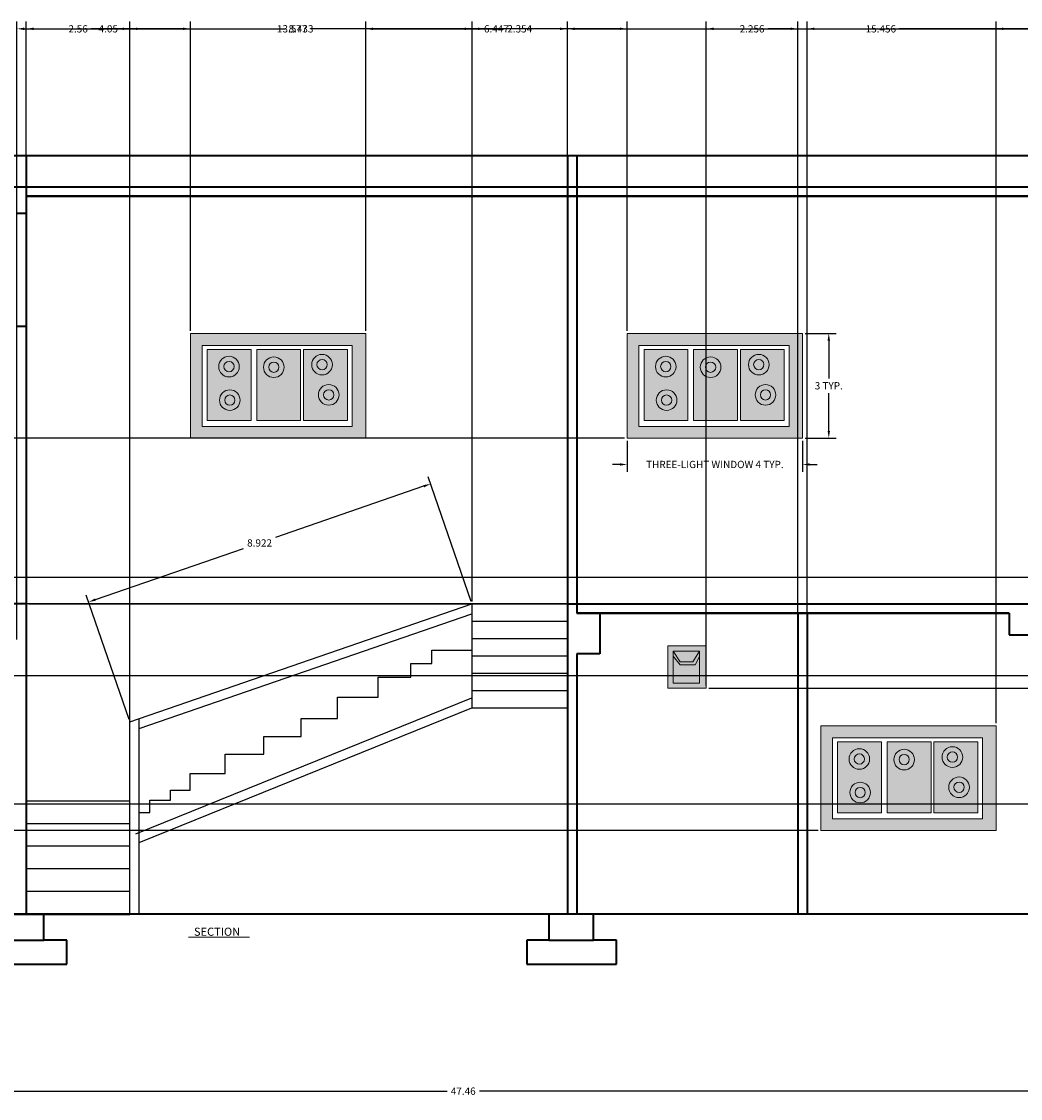
# Model space of a CAD drawing. Units: metres. Extents: x 1976.6 to 2045, y 823.7 to 850.3.
# Tile 2 of 3: x 2006.5 to 2031.2, y 823.7 to 850.3. Entities that reach past the tile are written whole.
import ezdxf

# ---------------------------------------------------------------- set-up
doc = ezdxf.new("R2010")
doc.units = ezdxf.units.M
for name, color, linetype, lineweight in [('A-ANNO-DIMS', 2, 'Continuous', 18), ('A-ANNO-TEXT', 7, 'Continuous', 18), ('A-COLS', 1, 'Continuous', 35), ('A-FLOR', 7, 'Continuous', 35), ('A-FLOR-STRS', 7, 'Continuous', 25), ('A-GLAZ', 4, 'Continuous', 18), ('A-ROOF', 7, 'Continuous', 35), ('A-WALL', 7, 'Continuous', 35), ('A-WALL-PRPT', 7, 'Continuous', 35), ('S-BEAM', 1, 'Continuous', 35), ('S-FNDN', 1, 'Continuous', 35)]:
    doc.layers.add(name, color=color, linetype=linetype, lineweight=lineweight)
doc.styles.get("Standard").update_dxf_attribs({"font": 'arial.ttf'})
doc.dimstyles.get("Standard").update_dxf_attribs({"dimtxt": 0.18, "dimasz": 0.18, "dimexe": 0.18, "dimexo": 0.0625, "dimgap": 0.09, "dimtad": 0, "dimtih": 1, "dimtoh": 1, "dimdec": 4, "dimzin": 0, "dimdsep": 46, "dimtxsty": 'Standard', "dimcen": 0.09, "dimadec": 0, "dimazin": 0, "dimtfac": 1, "dimtdec": 4, "dimtofl": 0, "dimtmove": 0, "dimatfit": 3, "dimfxl": 1, "dimtolj": 1, "dimtzin": 0, "dimarcsym": 0})

# ---------------------------------------------------------------- blocks, each defined once
blk = doc.blocks.new('WIN-THREE-LIGHT-ORNAMENTAL')
h = blk.add_hatch(color=256)
h.dxf.hatch_style = 1
h.paths.add_polyline_path([(4.324, 2.582), (0, 2.582), (0, 0), (4.324, 0)])
h.paths.add_polyline_path([(0.291, 2.284), (3.992, 2.284), (3.992, 0.289), (0.291, 0.289)], flags=16)
h.paths.add_polyline_path([(0.416, 2.189), (1.499, 2.189), (1.499, 0.436), (0.416, 0.436)], flags=0)
h.paths.add_polyline_path([(1.636, 2.189), (2.72, 2.189), (2.72, 0.436), (1.636, 0.436)], flags=0)
h.paths.add_polyline_path([(2.792, 2.189), (3.875, 2.189), (3.875, 0.436), (2.792, 0.436)], flags=0)
h = blk.add_hatch(color=256)
h.dxf.hatch_style = 1
h.paths.add_polyline_path([(1.499, 2.189), (0.416, 2.189), (0.416, 0.436), (1.499, 0.436)])
h.paths.add_polyline_path([(2.72, 2.189), (1.636, 2.189), (1.636, 0.436), (2.72, 0.436)])
h.paths.add_polyline_path([(3.875, 2.189), (2.792, 2.189), (2.792, 0.436), (3.875, 0.436)])
h = blk.add_hatch(color=256)
h.dxf.hatch_style = 1
h.paths.add_polyline_path([(1.207, 1.764, 1), (0.699, 1.764, 1)])
h.paths.add_polyline_path([(0.826, 1.764, -1), (1.08, 1.764, -1)], flags=16)
h = blk.add_hatch(color=256)
h.dxf.hatch_style = 1
h.paths.add_polyline_path([(2.312, 1.749, 1), (1.804, 1.749, 1)])
h.paths.add_polyline_path([(1.931, 1.749, -1), (2.186, 1.749, -1)], flags=16)
h = blk.add_hatch(color=256)
h.dxf.hatch_style = 1
h.paths.add_polyline_path([(3.501, 1.812, 1), (2.993, 1.812, 1)])
h.paths.add_polyline_path([(3.12, 1.812, -1), (3.374, 1.812, -1)], flags=16)
h = blk.add_hatch(color=256)
h.dxf.hatch_style = 1
h.paths.add_polyline_path([(1.227, 0.938, 1), (0.719, 0.938, 1)])
h.paths.add_polyline_path([(0.846, 0.938, -1), (1.1, 0.938, -1)], flags=16)
h = blk.add_hatch(color=256)
h.dxf.hatch_style = 1
h.paths.add_polyline_path([(2.366, 0.938, 1), (1.858, 0.938, 1)])
h.paths.add_polyline_path([(1.985, 0.938, -1), (2.239, 0.938, -1)], flags=16)
h = blk.add_hatch(color=256)
h.dxf.hatch_style = 1
h.paths.add_polyline_path([(3.666, 1.067, 1), (3.158, 1.067, 1)])
h.paths.add_polyline_path([(3.285, 1.067, -1), (3.539, 1.067, -1)], flags=16)
for points in [[(0, 2.582), (4.324, 2.582), (4.324, 0), (0, 0)], [(0.291, 2.284), (3.992, 2.284), (3.992, 0.289), (0.291, 0.289)], [(0.416, 2.189), (1.499, 2.189), (1.499, 0.436), (0.416, 0.436)], [(1.636, 2.189), (2.72, 2.189), (2.72, 0.436), (1.636, 0.436)], [(2.792, 2.189), (3.875, 2.189), (3.875, 0.436), (2.792, 0.436)]]:
    blk.add_lwpolyline(points, close=True)
for centre, radius in [((0.953, 1.764), 0.254), ((0.953, 1.764), 0.127), ((2.058, 1.749), 0.254), ((2.058, 1.749), 0.127), ((3.247, 1.812), 0.254), ((3.247, 1.812), 0.127), ((0.973, 0.938), 0.254), ((0.973, 0.938), 0.127), ((3.412, 1.067), 0.254), ((3.412, 1.067), 0.127)]:
    blk.add_circle(centre, radius)
blk = doc.blocks.new('WIN-VENT')
h = blk.add_hatch(color=256)
h.dxf.hatch_style = 1
h.paths.add_polyline_path([(0.783, 0.781), (0.783, 0.912), (0.616, 0.651), (0.305, 0.651), (0.133, 0.912), (0.133, 0.788), (0.305, 0.57), (0.677, 0.57)], flags=0)
h.paths.add_polyline_path([(0.95, 1.042), (0, 1.042), (0, 0), (0.95, 0)])
h.paths.add_polyline_path([(0.783, 0.912), (0.783, 0.125), (0.133, 0.125), (0.133, 0.912)], flags=16)
h.paths.add_polyline_path([(0.783, 0.781), (0.783, 0.912), (0.133, 0.912), (0.133, 0.788), (0.305, 0.57), (0.677, 0.57)], flags=0)
h = blk.add_hatch(color=256)
h.dxf.hatch_style = 1
h.paths.add_polyline_path([(0.783, 0.781), (0.783, 0.912), (0.616, 0.651), (0.305, 0.651), (0.133, 0.912), (0.133, 0.788), (0.305, 0.57), (0.677, 0.57)])
h = blk.add_hatch(color=256)
h.dxf.hatch_style = 1
h.paths.add_polyline_path([(0.133, 0.912), (0.305, 0.651), (0.616, 0.651), (0.783, 0.912)])
h.paths.add_polyline_path([(0.783, 0.125), (0.783, 0.781), (0.677, 0.57), (0.305, 0.57), (0.133, 0.788), (0.133, 0.125)])
for p, q in [((0.133, 0.912), (0.305, 0.651)), ((0.133, 0.912), (0.133, 0.788)), ((0.616, 0.651), (0.783, 0.912)), ((0.133, 0.788), (0.305, 0.57)), ((0.305, 0.651), (0.616, 0.651)), ((0.305, 0.57), (0.677, 0.57)), ((0.677, 0.57), (0.783, 0.781))]:
    blk.add_line(p, q)
for points in [[(0, 1.042), (0.95, 1.042), (0.95, 0), (0, 0)], [(0.133, 0.912), (0.783, 0.912), (0.783, 0.125), (0.133, 0.125)]]:
    blk.add_lwpolyline(points, close=True)
blk = doc.blocks.new('FNDN-STEPPED-PAD')
for p, q in [((0.547, 1.235), (0.547, 0.59)), ((1.641, 0.59), (1.641, 1.235)), ((0.547, 0.59), (0, 0.59)), ((0, 0.59), (0, 0)), ((0.547, 0.59), (1.641, 0.59)), ((2.209, 0.59), (1.641, 0.59)), ((2.209, 0), (2.209, 0.59)), ((0, 0), (2.209, 0))]:
    blk.add_line(p, q)
blk = doc.blocks.new('*D8')
at = {"layer": 'A-ANNO-DIMS', "color": 0, "lineweight": -2, "transparency": 16777216}
for p, q in [((2021.467, 839.959), (2021.467, 839.193)), ((2025.79, 839.959), (2025.79, 839.193)), ((2021.287, 839.373), (2021.107, 839.373)), ((2025.97, 839.373), (2026.15, 839.373))]:
    blk.add_line(p, q, dxfattribs=at)
at = {"layer": 'A-ANNO-DIMS', "color": 0, "transparency": 16777216}
for points in [[(2021.287, 839.403), (2021.287, 839.343), (2021.467, 839.373)], [(2025.97, 839.403), (2025.97, 839.343), (2025.79, 839.373)]]:
    blk.add_solid(points, dxfattribs=at)
at = {"layer": 'Defpoints', "color": 0, "transparency": 16777216}
for p in [(2021.467, 840.022), (2025.79, 840.022), (2025.79, 839.373)]:
    blk.add_point(p, dxfattribs=at)
at = {"layer": 'A-ANNO-DIMS', "color": 0, "transparency": 16777216, "insert": (2023.629, 839.373), "char_height": 0.18, "attachment_point": 5}
blk.add_mtext('\\A1;THREE-LIGHT WINDOW 4 TYP.', dxfattribs=at)
blk = doc.blocks.new('*D9')
at = {"layer": 'A-ANNO-DIMS', "color": 0, "lineweight": -2, "transparency": 16777216}
for p, q in [((2025.853, 842.604), (2026.619, 842.604)), ((2026.439, 842.424), (2026.439, 841.495)), ((2026.439, 840.202), (2026.439, 841.131)), ((2025.853, 840.022), (2026.619, 840.022))]:
    blk.add_line(p, q, dxfattribs=at)
at = {"layer": 'A-ANNO-DIMS', "color": 0, "transparency": 16777216}
for points in [[(2026.409, 842.424), (2026.469, 842.424), (2026.439, 842.604)], [(2026.409, 840.202), (2026.469, 840.202), (2026.439, 840.022)]]:
    blk.add_solid(points, dxfattribs=at)
at = {"layer": 'Defpoints', "color": 0, "transparency": 16777216}
for p in [(2025.79, 842.604), (2026.439, 842.604), (2025.79, 840.022)]:
    blk.add_point(p, dxfattribs=at)
at = {"layer": 'A-ANNO-DIMS', "color": 0, "transparency": 16777216, "insert": (2026.439, 841.313), "char_height": 0.18, "attachment_point": 5}
blk.add_mtext('\\A1;3 TYP.', dxfattribs=at)
blk = doc.blocks.new('*D16')
at = {"layer": 'A-ANNO-DIMS', "color": 0, "lineweight": -2, "transparency": 16777216}
for p, q in [((1993.695, 826.987), (1993.695, 823.74)), ((2041.154, 826.987), (2041.154, 823.74)), ((1993.875, 823.92), (2017.027, 823.92)), ((2040.974, 823.92), (2017.822, 823.92))]:
    blk.add_line(p, q, dxfattribs=at)
at = {"layer": 'A-ANNO-DIMS', "color": 0, "transparency": 16777216}
for points in [[(1993.875, 823.95), (1993.875, 823.89), (1993.695, 823.92)], [(2040.974, 823.95), (2040.974, 823.89), (2041.154, 823.92)]]:
    blk.add_solid(points, dxfattribs=at)
at = {"layer": 'Defpoints', "color": 0, "transparency": 16777216}
for p in [(1993.695, 827.05), (2041.154, 827.05), (2041.154, 823.92)]:
    blk.add_point(p, dxfattribs=at)
at = {"layer": 'A-ANNO-DIMS', "color": 0, "transparency": 16777216, "insert": (2017.425, 823.92), "char_height": 0.18, "attachment_point": 5}
blk.add_mtext('\\A1;47.46', dxfattribs=at)
blk = doc.blocks.new('*D20')
at = {"layer": 'A-ANNO-DIMS', "color": 0, "lineweight": -2, "transparency": 16777216}
for p, q in [((2006.418, 847.047), (2006.418, 850.295)), ((2019.995, 847.047), (2019.995, 850.295)), ((2006.598, 850.115), (2012.751, 850.115)), ((2019.815, 850.115), (2013.661, 850.115))]:
    blk.add_line(p, q, dxfattribs=at)
at = {"layer": 'A-ANNO-DIMS', "color": 0, "transparency": 16777216}
for points in [[(2006.598, 850.145), (2006.598, 850.085), (2006.418, 850.115)], [(2019.815, 850.145), (2019.815, 850.085), (2019.995, 850.115)]]:
    blk.add_solid(points, dxfattribs=at)
at = {"layer": 'Defpoints', "color": 0, "transparency": 16777216}
for p in [(2019.995, 850.115), (2006.418, 846.985), (2019.995, 846.985)]:
    blk.add_point(p, dxfattribs=at)
at = {"layer": 'A-ANNO-DIMS', "color": 0, "transparency": 16777216, "insert": (2013.206, 850.115), "char_height": 0.18, "attachment_point": 5}
blk.add_mtext('\\A1;13.577', dxfattribs=at)
blk = doc.blocks.new('*D21')
at = {"layer": 'A-ANNO-DIMS', "color": 0, "lineweight": -2, "transparency": 16777216}
for p, q in [((2019.995, 847.047), (2019.995, 850.295)), ((2035.451, 847.047), (2035.451, 850.295)), ((2020.175, 850.115), (2027.268, 850.115)), ((2035.271, 850.115), (2028.178, 850.115))]:
    blk.add_line(p, q, dxfattribs=at)
at = {"layer": 'A-ANNO-DIMS', "color": 0, "transparency": 16777216}
for points in [[(2020.175, 850.145), (2020.175, 850.085), (2019.995, 850.115)], [(2035.271, 850.145), (2035.271, 850.085), (2035.451, 850.115)]]:
    blk.add_solid(points, dxfattribs=at)
at = {"layer": 'Defpoints', "color": 0, "transparency": 16777216}
for p in [(2035.451, 850.115), (2019.995, 846.985), (2035.451, 846.985)]:
    blk.add_point(p, dxfattribs=at)
at = {"layer": 'A-ANNO-DIMS', "color": 0, "transparency": 16777216, "insert": (2027.723, 850.115), "char_height": 0.18, "attachment_point": 5}
blk.add_mtext('\\A1;15.456', dxfattribs=at)
blk = doc.blocks.new('*D23')
at = {"layer": 'A-ANNO-DIMS', "color": 0, "lineweight": -2, "transparency": 16777216}
for p, q in [((2006.71, 835.935), (2044.464, 835.935)), ((2044.284, 835.755), (2044.284, 832.292)), ((2044.284, 828.465), (2044.284, 831.928)), ((2006.71, 828.285), (2044.464, 828.285))]:
    blk.add_line(p, q, dxfattribs=at)
at = {"layer": 'A-ANNO-DIMS', "color": 0, "transparency": 16777216}
for points in [[(2044.254, 835.755), (2044.314, 835.755), (2044.284, 835.935)], [(2044.254, 828.465), (2044.314, 828.465), (2044.284, 828.285)]]:
    blk.add_solid(points, dxfattribs=at)
at = {"layer": 'Defpoints', "color": 0, "transparency": 16777216}
for p in [(2006.648, 835.935), (2044.284, 835.935), (2006.648, 828.285)]:
    blk.add_point(p, dxfattribs=at)
at = {"layer": 'A-ANNO-DIMS', "color": 0, "transparency": 16777216, "insert": (2044.284, 832.11), "char_height": 0.18, "attachment_point": 5}
blk.add_mtext('\\A1;7.65', dxfattribs=at)
blk = doc.blocks.new('*D26')
at = {"layer": 'A-ANNO-DIMS', "color": 0, "lineweight": -2, "transparency": 16777216}
for p, q in [((2006.648, 828.347), (2006.648, 850.295)), ((2009.207, 828.347), (2009.207, 850.295)), ((2006.828, 850.115), (2007.602, 850.115)), ((2009.027, 850.115), (2008.253, 850.115))]:
    blk.add_line(p, q, dxfattribs=at)
at = {"layer": 'A-ANNO-DIMS', "color": 0, "transparency": 16777216}
for points in [[(2006.828, 850.145), (2006.828, 850.085), (2006.648, 850.115)], [(2009.027, 850.145), (2009.027, 850.085), (2009.207, 850.115)]]:
    blk.add_solid(points, dxfattribs=at)
at = {"layer": 'Defpoints', "color": 0, "transparency": 16777216}
for p in [(2009.207, 850.115), (2006.648, 828.285), (2009.207, 828.285)]:
    blk.add_point(p, dxfattribs=at)
at = {"layer": 'A-ANNO-DIMS', "color": 0, "transparency": 16777216, "insert": (2007.928, 850.115), "char_height": 0.18, "attachment_point": 5}
blk.add_mtext('\\A1;2.56', dxfattribs=at)
blk = doc.blocks.new('*D27')
at = {"layer": 'A-ANNO-DIMS', "color": 0, "lineweight": -2, "transparency": 16777216}
for p, q in [((2009.207, 833.086), (2009.207, 850.295)), ((2017.641, 835.997), (2017.641, 850.295)), ((2009.387, 850.115), (2013.03, 850.115)), ((2017.461, 850.115), (2013.818, 850.115))]:
    blk.add_line(p, q, dxfattribs=at)
at = {"layer": 'A-ANNO-DIMS', "color": 0, "transparency": 16777216}
for points in [[(2009.387, 850.145), (2009.387, 850.085), (2009.207, 850.115)], [(2017.461, 850.145), (2017.461, 850.085), (2017.641, 850.115)]]:
    blk.add_solid(points, dxfattribs=at)
at = {"layer": 'Defpoints', "color": 0, "transparency": 16777216}
for p in [(2017.641, 850.115), (2017.641, 835.935), (2009.207, 833.023)]:
    blk.add_point(p, dxfattribs=at)
at = {"layer": 'A-ANNO-DIMS', "color": 0, "transparency": 16777216, "insert": (2013.424, 850.115), "char_height": 0.18, "attachment_point": 5}
blk.add_mtext('\\A1;8.433', dxfattribs=at)
blk = doc.blocks.new('*D28')
at = {"layer": 'A-ANNO-DIMS', "color": 0, "lineweight": -2, "transparency": 16777216}
for p, q in [((2017.62, 835.994), (2016.561, 839.064)), ((2016.449, 838.835), (2012.796, 837.573)), ((2008.356, 836.041), (2012.01, 837.302)), ((2009.187, 833.082), (2008.127, 836.152))]:
    blk.add_line(p, q, dxfattribs=at)
at = {"layer": 'A-ANNO-DIMS', "color": 0, "transparency": 16777216}
for points in [[(2016.439, 838.863), (2016.459, 838.806), (2016.619, 838.893)], [(2008.346, 836.069), (2008.366, 836.012), (2008.186, 835.982)]]:
    blk.add_solid(points, dxfattribs=at)
at = {"layer": 'Defpoints', "color": 0, "transparency": 16777216}
for p in [(2016.619, 838.893), (2017.641, 835.935), (2009.207, 833.023)]:
    blk.add_point(p, dxfattribs=at)
at = {"layer": 'A-ANNO-DIMS', "color": 0, "transparency": 16777216, "insert": (2012.403, 837.438), "char_height": 0.18, "attachment_point": 5}
blk.add_mtext('\\A1;8.922', dxfattribs=at)
blk = doc.blocks.new('*D29')
at = {"layer": 'A-ANNO-DIMS', "color": 0, "lineweight": -2, "transparency": 16777216}
for p, q in [((2017.641, 835.997), (2017.641, 850.295)), ((2019.995, 835.997), (2019.995, 850.295)), ((2017.821, 850.115), (2018.423, 850.115)), ((2019.815, 850.115), (2019.213, 850.115))]:
    blk.add_line(p, q, dxfattribs=at)
at = {"layer": 'A-ANNO-DIMS', "color": 0, "transparency": 16777216}
for points in [[(2017.821, 850.145), (2017.821, 850.085), (2017.641, 850.115)], [(2019.815, 850.145), (2019.815, 850.085), (2019.995, 850.115)]]:
    blk.add_solid(points, dxfattribs=at)
at = {"layer": 'Defpoints', "color": 0, "transparency": 16777216}
for p in [(2019.995, 850.115), (2017.641, 835.935), (2019.995, 835.935)]:
    blk.add_point(p, dxfattribs=at)
at = {"layer": 'A-ANNO-DIMS', "color": 0, "transparency": 16777216, "insert": (2018.818, 850.115), "char_height": 0.18, "attachment_point": 5}
blk.add_mtext('\\A1;2.354', dxfattribs=at)
blk = doc.blocks.new('*D30')
at = {"layer": 'A-ANNO-DIMS', "color": 0, "lineweight": -2, "transparency": 16777216}
for p, q in [((2025.906, 828.347), (2025.906, 850.295)), ((2039.878, 828.347), (2039.878, 850.295)), ((2026.086, 850.115), (2032.437, 850.115)), ((2039.698, 850.115), (2033.346, 850.115))]:
    blk.add_line(p, q, dxfattribs=at)
at = {"layer": 'A-ANNO-DIMS', "color": 0, "transparency": 16777216}
for points in [[(2026.086, 850.145), (2026.086, 850.085), (2025.906, 850.115)], [(2039.698, 850.145), (2039.698, 850.085), (2039.878, 850.115)]]:
    blk.add_solid(points, dxfattribs=at)
at = {"layer": 'Defpoints', "color": 0, "transparency": 16777216}
for p in [(2039.878, 850.115), (2025.906, 828.285), (2039.878, 828.285)]:
    blk.add_point(p, dxfattribs=at)
at = {"layer": 'A-ANNO-DIMS', "color": 0, "transparency": 16777216, "insert": (2032.892, 850.115), "char_height": 0.18, "attachment_point": 5}
blk.add_mtext('\\A1;13.972', dxfattribs=at)
blk = doc.blocks.new('*D32')
at = {"layer": 'A-ANNO-DIMS', "color": 0, "lineweight": -2, "transparency": 16777216}
for p, q in [((1997.363, 831.006), (2044.464, 831.006)), ((2044.284, 830.826), (2044.284, 829.826)), ((2044.284, 828.465), (2044.284, 829.465)), ((1994.937, 828.285), (2044.464, 828.285))]:
    blk.add_line(p, q, dxfattribs=at)
at = {"layer": 'A-ANNO-DIMS', "color": 0, "transparency": 16777216}
for points in [[(2044.254, 830.826), (2044.314, 830.826), (2044.284, 831.006)], [(2044.254, 828.465), (2044.314, 828.465), (2044.284, 828.285)]]:
    blk.add_solid(points, dxfattribs=at)
at = {"layer": 'Defpoints', "color": 0, "transparency": 16777216}
for p in [(1997.3, 831.006), (1994.875, 828.285), (2044.284, 828.285)]:
    blk.add_point(p, dxfattribs=at)
at = {"layer": 'A-ANNO-DIMS', "color": 0, "transparency": 16777216, "insert": (2044.284, 829.645), "char_height": 0.18, "attachment_point": 5}
blk.add_mtext('\\A1;2.721', dxfattribs=at)
blk = doc.blocks.new('*D36')
at = {"layer": 'A-ANNO-DIMS', "color": 0, "lineweight": -2, "transparency": 16777216}
for p, q in [((2005.307, 834.228), (2005.307, 850.295)), ((2006.418, 835.06), (2006.418, 850.295)), ((2005.127, 850.115), (2004.947, 850.115)), ((2006.598, 850.115), (2006.778, 850.115))]:
    blk.add_line(p, q, dxfattribs=at)
at = {"layer": 'A-ANNO-DIMS', "color": 0, "transparency": 16777216}
for points in [[(2005.127, 850.145), (2005.127, 850.085), (2005.307, 850.115)], [(2006.598, 850.145), (2006.598, 850.085), (2006.418, 850.115)]]:
    blk.add_solid(points, dxfattribs=at)
at = {"layer": 'Defpoints', "color": 0, "transparency": 16777216}
for p in [(2006.418, 850.115), (2006.418, 834.998), (2005.307, 834.166)]:
    blk.add_point(p, dxfattribs=at)
at = {"layer": 'A-ANNO-DIMS', "color": 0, "transparency": 16777216, "insert": (2005.862, 850.115), "char_height": 0.18, "attachment_point": 5}
blk.add_mtext('\\A1;1.11', dxfattribs=at)
blk = doc.blocks.new('*D38')
at = {"layer": 'A-ANNO-DIMS', "color": 0, "lineweight": -2, "transparency": 16777216}
for p, q in [((2005.369, 834.166), (2044.464, 834.166)), ((2044.284, 833.986), (2044.284, 831.407)), ((2044.284, 828.465), (2044.284, 831.043)), ((2005.369, 828.285), (2044.464, 828.285))]:
    blk.add_line(p, q, dxfattribs=at)
at = {"layer": 'A-ANNO-DIMS', "color": 0, "transparency": 16777216}
for points in [[(2044.254, 833.986), (2044.314, 833.986), (2044.284, 834.166)], [(2044.254, 828.465), (2044.314, 828.465), (2044.284, 828.285)]]:
    blk.add_solid(points, dxfattribs=at)
at = {"layer": 'Defpoints', "color": 0, "transparency": 16777216}
for p in [(2005.307, 834.166), (2005.307, 828.285), (2044.284, 828.285)]:
    blk.add_point(p, dxfattribs=at)
at = {"layer": 'A-ANNO-DIMS', "color": 0, "transparency": 16777216, "insert": (2044.284, 831.225), "char_height": 0.18, "attachment_point": 5}
blk.add_mtext('\\A1;5.881', dxfattribs=at)
blk = doc.blocks.new('*D39')
at = {"layer": 'A-ANNO-DIMS', "color": 0, "lineweight": -2, "transparency": 16777216}
for p, q in [((2006.648, 842.847), (2006.648, 850.295)), ((2010.696, 842.666), (2010.696, 850.295)), ((2006.828, 850.115), (2008.344, 850.115)), ((2010.516, 850.115), (2009, 850.115))]:
    blk.add_line(p, q, dxfattribs=at)
at = {"layer": 'A-ANNO-DIMS', "color": 0, "transparency": 16777216}
for points in [[(2006.828, 850.145), (2006.828, 850.085), (2006.648, 850.115)], [(2010.516, 850.145), (2010.516, 850.085), (2010.696, 850.115)]]:
    blk.add_solid(points, dxfattribs=at)
at = {"layer": 'Defpoints', "color": 0, "transparency": 16777216}
for p in [(2010.696, 850.115), (2006.648, 842.785), (2010.696, 842.604)]:
    blk.add_point(p, dxfattribs=at)
at = {"layer": 'A-ANNO-DIMS', "color": 0, "transparency": 16777216, "insert": (2008.672, 850.115), "char_height": 0.18, "attachment_point": 5}
blk.add_mtext('\\A1;4.05', dxfattribs=at)
blk = doc.blocks.new('*D40')
at = {"layer": 'A-ANNO-DIMS', "color": 0, "lineweight": -2, "transparency": 16777216}
for p, q in [((2015.02, 842.666), (2015.02, 850.295)), ((2021.467, 842.666), (2021.467, 850.295)), ((2015.2, 850.115), (2017.849, 850.115)), ((2021.287, 850.115), (2018.638, 850.115))]:
    blk.add_line(p, q, dxfattribs=at)
at = {"layer": 'A-ANNO-DIMS', "color": 0, "transparency": 16777216}
for points in [[(2015.2, 850.145), (2015.2, 850.085), (2015.02, 850.115)], [(2021.287, 850.145), (2021.287, 850.085), (2021.467, 850.115)]]:
    blk.add_solid(points, dxfattribs=at)
at = {"layer": 'Defpoints', "color": 0, "transparency": 16777216}
for p in [(2021.467, 850.115), (2015.02, 842.604), (2021.467, 842.604)]:
    blk.add_point(p, dxfattribs=at)
at = {"layer": 'A-ANNO-DIMS', "color": 0, "transparency": 16777216, "insert": (2018.243, 850.115), "char_height": 0.18, "attachment_point": 5}
blk.add_mtext('\\A1;6.447', dxfattribs=at)
blk = doc.blocks.new('*D41')
at = {"layer": 'A-ANNO-DIMS', "color": 0, "lineweight": -2, "transparency": 16777216}
for p, q in [((2026.178, 830.345), (1986.237, 830.345)), ((1986.417, 830.165), (1986.417, 829.497)), ((1986.417, 828.465), (1986.417, 829.133)), ((2025.843, 828.285), (1986.237, 828.285))]:
    blk.add_line(p, q, dxfattribs=at)
at = {"layer": 'A-ANNO-DIMS', "color": 0, "transparency": 16777216}
for points in [[(1986.387, 830.165), (1986.447, 830.165), (1986.417, 830.345)], [(1986.387, 828.465), (1986.447, 828.465), (1986.417, 828.285)]]:
    blk.add_solid(points, dxfattribs=at)
at = {"layer": 'Defpoints', "color": 0, "transparency": 16777216}
for p in [(2026.24, 830.345), (1986.417, 828.285), (2025.906, 828.285)]:
    blk.add_point(p, dxfattribs=at)
at = {"layer": 'A-ANNO-DIMS', "color": 0, "transparency": 16777216, "insert": (1986.417, 829.315), "char_height": 0.18, "attachment_point": 5}
blk.add_mtext('\\A1;2.06', dxfattribs=at)
blk = doc.blocks.new('*D42')
at = {"layer": 'A-ANNO-DIMS', "color": 0, "lineweight": -2, "transparency": 16777216}
for p, q in [((2021.404, 840.022), (1986.237, 840.022)), ((1986.417, 839.842), (1986.417, 838.16)), ((1986.417, 836.115), (1986.417, 837.796)), ((2020.162, 835.935), (1986.237, 835.935))]:
    blk.add_line(p, q, dxfattribs=at)
at = {"layer": 'A-ANNO-DIMS', "color": 0, "transparency": 16777216}
for points in [[(1986.387, 839.842), (1986.447, 839.842), (1986.417, 840.022)], [(1986.387, 836.115), (1986.447, 836.115), (1986.417, 835.935)]]:
    blk.add_solid(points, dxfattribs=at)
at = {"layer": 'Defpoints', "color": 0, "transparency": 16777216}
for p in [(2021.467, 840.022), (1986.417, 835.935), (2020.225, 835.935)]:
    blk.add_point(p, dxfattribs=at)
at = {"layer": 'A-ANNO-DIMS', "color": 0, "transparency": 16777216, "insert": (1986.417, 837.978), "char_height": 0.18, "attachment_point": 5}
blk.add_mtext('\\A1;4.087', dxfattribs=at)
blk = doc.blocks.new('*D43')
at = {"layer": 'A-ANNO-DIMS', "color": 0, "lineweight": -2, "transparency": 16777216}
for p, q in [((2030.564, 832.99), (2030.564, 850.295)), ((2039.878, 832.797), (2039.878, 850.295)), ((2030.744, 850.115), (2034.827, 850.115)), ((2039.698, 850.115), (2035.614, 850.115))]:
    blk.add_line(p, q, dxfattribs=at)
at = {"layer": 'A-ANNO-DIMS', "color": 0, "transparency": 16777216}
for points in [[(2030.744, 850.145), (2030.744, 850.085), (2030.564, 850.115)], [(2039.698, 850.145), (2039.698, 850.085), (2039.878, 850.115)]]:
    blk.add_solid(points, dxfattribs=at)
at = {"layer": 'Defpoints', "color": 0, "transparency": 16777216}
for p in [(2039.878, 850.115), (2030.564, 832.927), (2039.878, 832.735)]:
    blk.add_point(p, dxfattribs=at)
at = {"layer": 'A-ANNO-DIMS', "color": 0, "transparency": 16777216, "insert": (2035.221, 850.115), "char_height": 0.18, "attachment_point": 5}
blk.add_mtext('\\A1;9.314', dxfattribs=at)
blk = doc.blocks.new('*D46')
at = {"layer": 'A-ANNO-DIMS', "color": 0, "lineweight": -2, "transparency": 16777216}
for p, q in [((2023.419, 833.921), (2023.419, 850.295)), ((2025.676, 828.347), (2025.676, 850.295)), ((2023.599, 850.115), (2024.152, 850.115)), ((2025.496, 850.115), (2024.943, 850.115))]:
    blk.add_line(p, q, dxfattribs=at)
at = {"layer": 'A-ANNO-DIMS', "color": 0, "transparency": 16777216}
for points in [[(2023.599, 850.145), (2023.599, 850.085), (2023.419, 850.115)], [(2025.496, 850.145), (2025.496, 850.085), (2025.676, 850.115)]]:
    blk.add_solid(points, dxfattribs=at)
at = {"layer": 'Defpoints', "color": 0, "transparency": 16777216}
for p in [(2025.676, 850.115), (2023.419, 833.859), (2025.676, 828.285)]:
    blk.add_point(p, dxfattribs=at)
at = {"layer": 'A-ANNO-DIMS', "color": 0, "transparency": 16777216, "insert": (2024.547, 850.115), "char_height": 0.18, "attachment_point": 5}
blk.add_mtext('\\A1;2.256', dxfattribs=at)
blk = doc.blocks.new('*D47')
at = {"layer": 'A-ANNO-DIMS', "color": 0, "lineweight": -2, "transparency": 16777216}
for p, q in [((2023.482, 833.859), (2044.464, 833.859)), ((2044.284, 833.679), (2044.284, 831.253)), ((2044.284, 828.465), (2044.284, 830.89)), ((2025.738, 828.285), (2044.464, 828.285))]:
    blk.add_line(p, q, dxfattribs=at)
at = {"layer": 'A-ANNO-DIMS', "color": 0, "transparency": 16777216}
for points in [[(2044.254, 833.679), (2044.314, 833.679), (2044.284, 833.859)], [(2044.254, 828.465), (2044.314, 828.465), (2044.284, 828.285)]]:
    blk.add_solid(points, dxfattribs=at)
at = {"layer": 'Defpoints', "color": 0, "transparency": 16777216}
for p in [(2023.419, 833.859), (2025.676, 828.285), (2044.284, 828.285)]:
    blk.add_point(p, dxfattribs=at)
at = {"layer": 'A-ANNO-DIMS', "color": 0, "transparency": 16777216, "insert": (2044.284, 831.072), "char_height": 0.18, "attachment_point": 5}
blk.add_mtext('\\A1;5.574', dxfattribs=at)
blk = doc.blocks.new('*D48')
at = {"layer": 'A-ANNO-DIMS', "color": 0, "lineweight": -2, "transparency": 16777216}
for p, q in [((2038.162, 836.589), (1986.237, 836.589)), ((1986.417, 836.409), (1986.417, 836.115)), ((2039.726, 835.935), (1986.237, 835.935)), ((1986.417, 835.755), (1986.237, 835.755)), ((1986.417, 835.935), (1986.417, 835.755))]:
    blk.add_line(p, q, dxfattribs=at)
at = {"layer": 'A-ANNO-DIMS', "color": 0, "transparency": 16777216}
for points in [[(1986.387, 836.409), (1986.447, 836.409), (1986.417, 836.589)], [(1986.387, 836.115), (1986.447, 836.115), (1986.417, 835.935)]]:
    blk.add_solid(points, dxfattribs=at)
at = {"layer": 'Defpoints', "color": 0, "transparency": 16777216}
for p in [(2038.224, 836.589), (1986.417, 835.935), (2039.788, 835.935)]:
    blk.add_point(p, dxfattribs=at)
at = {"layer": 'A-ANNO-DIMS', "color": 0, "transparency": 16777216, "insert": (1985.913, 835.755), "char_height": 0.18, "attachment_point": 5}
blk.add_mtext('\\A1;0.65', dxfattribs=at)

msp = doc.modelspace()

# ---------------------------------------------------------------- linework, layer by layer
at = {"layer": 'A-ANNO-TEXT'}
msp.add_line((2010.654, 827.7207), (2012.1564, 827.7207), dxfattribs=at)
at = {"layer": 'A-COLS'}
for p, q in [((2006.6479, 846.9848), (2006.6479, 835.9348)), ((2019.9947, 846.9848), (2019.9947, 835.9348)), ((2020.2247, 846.9848), (2020.2247, 835.9348)), ((2006.4179, 842.7848), (2006.6479, 842.7848)), ((2006.6479, 835.9348), (2006.6479, 828.2848)), ((2019.9947, 835.9348), (2019.9947, 828.2848)), ((2020.2247, 835.9348), (2020.2247, 835.7048)), ((2020.2247, 834.7023), (2020.2247, 828.2848))]:
    msp.add_line(p, q, dxfattribs=at)
at = {"layer": 'A-FLOR'}
for p, q in [((2006.6479, 835.9348), (1993.6952, 835.9348)), ((2019.9947, 835.9348), (2040.0184, 835.9348)), ((2020.2247, 835.7048), (2030.8908, 835.7048)), ((2020.2247, 835.7048), (2025.6756, 835.7048)), ((2020.2247, 835.7048), (2030.8908, 835.7048)), ((2030.8908, 835.7048), (2020.2247, 835.7048)), ((2040.5852, 828.2848), (1993.0497, 828.2848)), ((2040.5852, 828.2848), (1994.6446, 828.2848)), ((1994.6446, 828.2848), (2009.2074, 828.2848))]:
    msp.add_line(p, q, dxfattribs=at)
at = {"layer": 'A-FLOR-STRS'}
for p, q in [((2009.2074, 833.0232), (2017.6409, 835.9348)), ((2009.4374, 832.8593), (2017.6409, 835.6915)), ((2019.9947, 835.9348), (2017.6409, 835.9348)), ((2017.6409, 835.9348), (2017.6409, 834.0079)), ((2017.6409, 835.9348), (2019.9947, 835.9348)), ((2017.6409, 835.5072), (2019.9947, 835.5072)), ((2017.6409, 835.0795), (2019.9947, 835.0795)), ((2016.6543, 834.4682), (2016.6543, 834.794)), ((2016.6543, 834.794), (2017.6409, 834.794)), ((2017.6409, 834.6519), (2019.9947, 834.6519)), ((2016.1349, 834.1242), (2016.1349, 834.4682)), ((2016.1349, 834.4682), (2016.6543, 834.4682)), ((2015.3254, 833.6315), (2015.3254, 834.1242)), ((2015.3254, 834.1242), (2016.1349, 834.1242)), ((2017.6409, 834.2242), (2019.9947, 834.2242)), ((2017.6409, 834.0079), (2017.6409, 833.3689)), ((2009.3511, 830.2635), (2017.6409, 833.617)), ((2014.3265, 833.1102), (2014.3265, 833.6315)), ((2014.3265, 833.6315), (2015.3254, 833.6315)), ((2017.6409, 833.7966), (2019.9947, 833.7966)), ((2009.4374, 830.0503), (2017.6409, 833.3689)), ((2017.6409, 833.3689), (2019.9947, 833.3689)), ((2017.6409, 833.3689), (2019.9947, 833.3689)), ((2009.4374, 831.0722), (2009.4374, 833.1026)), ((2013.4319, 832.6633), (2013.4319, 833.1102)), ((2013.4319, 833.1102), (2014.3265, 833.1102)), ((2009.2074, 831.0722), (2009.2074, 833.0232)), ((2012.5075, 832.2313), (2012.5075, 832.6633)), ((2012.5075, 832.6633), (2013.4319, 832.6633)), ((2011.5533, 831.7546), (2011.5533, 832.2313)), ((2011.5533, 832.2313), (2012.5075, 832.2313)), ((2010.6924, 831.3434), (2010.6924, 831.7546)), ((2010.6924, 831.7546), (2011.5533, 831.7546)), ((2010.2088, 831.0931), (2010.2088, 831.3434)), ((2010.2088, 831.3434), (2010.6924, 831.3434)), ((2009.2074, 831.0722), (2006.6479, 831.0722)), ((2009.2074, 831.0722), (2008.9769, 831.0722)), ((2009.2074, 830.984), (2009.2074, 831.0722)), ((2009.2074, 828.2848), (2009.2074, 830.984)), ((2009.4374, 828.2848), (2009.4374, 831.0722)), ((2009.4374, 830.2984), (2009.4374, 831.0722)), ((2009.6963, 830.7879), (2009.6963, 831.0931)), ((2009.6963, 831.0931), (2010.2088, 831.0931)), ((2009.4374, 830.2984), (2009.4374, 830.7879)), ((2009.4374, 830.7879), (2009.6963, 830.7879)), ((2009.2074, 830.5147), (2006.6479, 830.5147)), ((2009.2074, 829.9572), (2006.6479, 829.9572)), ((2009.2074, 829.3998), (2009.2074, 829.9572)), ((2009.2074, 829.3998), (2006.6479, 829.3998)), ((2009.2074, 828.8423), (2006.6479, 828.8423)), ((2009.2074, 828.2848), (2006.6479, 828.2848))]:
    msp.add_line(p, q, dxfattribs=at)
at = {"layer": 'A-ROOF'}
for p, q in [((2040.0184, 846.2148), (1993.6952, 846.2148)), ((2006.6479, 845.9848), (2040.0184, 845.9848)), ((2040.0184, 845.9848), (2006.6479, 845.9848))]:
    msp.add_line(p, q, dxfattribs=at)
at = {"layer": 'A-WALL'}
for p, q in [((2025.6756, 835.7048), (2025.6756, 828.2848)), ((2025.9056, 835.7048), (2025.9056, 828.2848))]:
    msp.add_line(p, q, dxfattribs=at)
at = {"layer": 'A-WALL-PRPT'}
msp.add_line((2040.0184, 846.9848), (1994.6446, 846.9848), dxfattribs=at)
at = {"layer": 'S-BEAM'}
for p, q in [((2006.4179, 845.5737), (2006.6479, 845.5737)), ((2020.79, 835.7048), (2020.79, 834.7023)), ((2030.8908, 835.7048), (2030.8908, 835.1735)), ((2030.8908, 835.1735), (2031.4404, 835.1735)), ((2020.79, 834.7023), (2020.2247, 834.7023))]:
    msp.add_line(p, q, dxfattribs=at)

# ---------------------------------------------------------------- block references
at = {"layer": 'A-GLAZ'}
for name, p in [('WIN-THREE-LIGHT-ORNAMENTAL', (2010.696, 840.022)), ('WIN-THREE-LIGHT-ORNAMENTAL', (2021.4665, 840.022)), ('WIN-VENT', (2022.4693, 833.8591)), ('WIN-THREE-LIGHT-ORNAMENTAL', (2026.2399, 830.3457))]:
    msp.add_blockref(name, p, dxfattribs=at)
at = {"layer": 'S-FNDN'}
for p in [(2005.4419, 827.05), (2018.9927, 827.05)]:
    msp.add_blockref('FNDN-STEPPED-PAD', p, dxfattribs=at)

# ---------------------------------------------------------------- texts
at = {"layer": 'A-ANNO-TEXT', "insert": (2010.784, 828.2848), "char_height": 0.2, "attachment_point": 1}
msp.add_mtext_dynamic_manual_height_columns('\\PSECTION', width=3.952793, gutter_width=12.5, heights=[0], dxfattribs=at)

# ---------------------------------------------------------------- dimensions: what is measured, and where the dimension line sits
at = {"layer": 'A-ANNO-DIMS'}
for base, p1, p2, override, picture, middle in [((2006.4179, 850.1148), (2005.3067, 834.1656), (2006.4179, 834.9975), {"dimdec": 2, "dimlfac": 1, "dimrnd": 0, "dimzin": 0, "dimdsep": 46, "dimlunit": 2}, '*D36', (2005.8623, 850.1148)), ((2019.9947, 850.1148), (2006.4179, 846.9848), (2019.9947, 846.9848), {"dimdec": 3, "dimlfac": 1, "dimrnd": 0, "dimzin": 0, "dimdsep": 46, "dimlunit": 2}, '*D20', (2013.2063, 850.1148)), ((2009.2074, 850.1148), (2006.6479, 828.2848), (2009.2074, 828.2848), {"dimdec": 2, "dimlfac": 1, "dimrnd": 0, "dimzin": 0, "dimdsep": 46, "dimlunit": 2}, '*D26', (2007.9277, 850.1148)), ((2010.6964, 850.1148), (2006.6479, 842.7848), (2010.6964, 842.6036), {"dimdec": 2, "dimlfac": 1, "dimrnd": 0, "dimzin": 0, "dimdsep": 46, "dimlunit": 2}, '*D39', (2008.6722, 850.1148)), ((2017.64087, 850.11482), (2009.2074, 833.0232), (2017.64087, 835.93482), {"dimdec": 3, "dimlfac": 1, "dimrnd": 0, "dimzin": 0, "dimdsep": 46, "dimlunit": 2}, '*D27', (2013.42413, 850.11482)), ((2021.4669, 850.1148), (2015.02, 842.6036), (2021.4669, 842.6036), {"dimdec": 3, "dimlfac": 1, "dimrnd": 0, "dimzin": 0, "dimdsep": 46, "dimlunit": 2}, '*D40', (2018.2435, 850.1148)), ((2019.9947, 850.1148), (2017.6409, 835.9348), (2019.9947, 835.9348), {"dimdec": 3, "dimlfac": 1, "dimrnd": 0, "dimzin": 0, "dimdsep": 46, "dimlunit": 2}, '*D29', (2018.8178, 850.1148)), ((2035.4511, 850.1148), (2019.9947, 846.9848), (2035.4511, 846.9848), {"dimdec": 3, "dimlfac": 1, "dimrnd": 0, "dimzin": 0, "dimdsep": 46, "dimlunit": 2}, '*D21', (2027.7229, 850.1148)), ((2025.6756, 850.1148), (2023.4194, 833.8587), (2025.6756, 828.2848), {"dimdec": 3, "dimlfac": 1, "dimrnd": 0, "dimzin": 0, "dimdsep": 46, "dimlunit": 2}, '*D46', (2024.5475, 850.1148)), ((2039.8775, 850.1148), (2025.9056, 828.2848), (2039.8775, 828.2848), {"dimdec": 3, "dimlfac": 1, "dimrnd": 0, "dimzin": 0, "dimdsep": 46, "dimlunit": 2}, '*D30', (2032.8915, 850.1148)), ((2039.8775, 850.1148), (2030.5639, 832.9273), (2039.8775, 832.7348), {"dimdec": 3, "dimlfac": 1, "dimrnd": 0, "dimzin": 0, "dimdsep": 46, "dimlunit": 2}, '*D43', (2035.2207, 850.1148)), ((2041.1538, 823.9197), (1993.6952, 827.0497), (2041.1538, 827.0497), {"dimdec": 2, "dimlfac": 1, "dimrnd": 0, "dimzin": 0, "dimdsep": 46, "dimlunit": 2}, '*D16', (2017.4245, 823.9197))]:
    dim = msp.add_linear_dim(base=base, p1=p1, p2=p2, dimstyle='Standard', override=override, dxfattribs=at)
    dim.commit()
    dim.dimension.update_dxf_attribs({"geometry": picture, "text_midpoint": middle})
dim = msp.add_linear_dim(base=(2026.439, 842.6036), p1=(2025.7905, 840.0217), p2=(2025.7905, 842.6036), angle=90, text='<> TYP.', dimstyle='Standard', override={"dimdec": 0, "dimlfac": 1, "dimrnd": 0, "dimzin": 0, "dimdsep": 46, "dimlunit": 2}, dxfattribs=at)
dim.commit()
dim.dimension.update_dxf_attribs({"geometry": '*D9', "text_midpoint": (2026.439, 841.3126)})
for base, p1, p2, angle, override, picture, middle in [((1986.4174, 835.9348), (2021.4669, 840.0217), (2020.2247, 835.9348), 90, {"dimdec": 3, "dimlfac": 1, "dimrnd": 0, "dimzin": 0, "dimdsep": 46, "dimlunit": 2}, '*D42', (1986.4174, 837.9782)), ((2016.6194, 838.8935), (2009.2074, 833.0232), (2017.6409, 835.9348), 19.04697, {"dimdec": 3, "dimlfac": 1, "dimrnd": 0, "dimzin": 0, "dimdsep": 46, "dimlunit": 2}, '*D28', (2012.4027, 837.4376)), ((1986.4174, 835.9348), (2038.2243, 836.5887), (2039.7884, 835.9348), 90, {"dimdec": 2, "dimlfac": 1, "dimrnd": 0, "dimzin": 0, "dimdsep": 46, "dimlunit": 2}, '*D48', (1985.913, 835.7548)), ((2044.2838, 835.9348), (2006.6479, 828.2848), (2006.6479, 835.9348), 90, {"dimdec": 2, "dimlfac": 1, "dimrnd": 0, "dimzin": 0, "dimdsep": 46, "dimlunit": 2}, '*D23', (2044.2838, 832.1098)), ((2044.2838, 828.2848), (2005.3067, 834.1656), (2005.3067, 828.2848), 90, {"dimdec": 3, "dimlfac": 1, "dimrnd": 0, "dimzin": 0, "dimdsep": 46, "dimlunit": 2}, '*D38', (2044.2838, 831.2252)), ((2044.2838, 828.2848), (2023.4194, 833.8587), (2025.6756, 828.2848), 90, {"dimdec": 3, "dimlfac": 1, "dimrnd": 0, "dimzin": 0, "dimdsep": 46, "dimlunit": 2}, '*D47', (2044.2838, 831.0718)), ((2044.2838, 828.2848), (1997.3001, 831.0057), (1994.8746, 828.2848), 90, {"dimdec": 3, "dimlfac": 1, "dimrnd": 0, "dimzin": 0, "dimdsep": 46, "dimlunit": 2}, '*D32', (2044.2838, 829.6453)), ((1986.4174, 828.2848), (2026.2403, 830.3453), (2025.9056, 828.2848), 90, {"dimdec": 2, "dimlfac": 1, "dimrnd": 0, "dimzin": 0, "dimdsep": 46, "dimlunit": 2}, '*D41', (1986.4174, 829.3151))]:
    dim = msp.add_linear_dim(base=base, p1=p1, p2=p2, angle=angle, dimstyle='Standard', override=override, dxfattribs=at)
    dim.commit()
    dim.dimension.update_dxf_attribs({"geometry": picture, "text_midpoint": middle})
dim = msp.add_linear_dim(base=(2025.7905, 839.3731), p1=(2021.4669, 840.0217), p2=(2025.7905, 840.0217), text='THREE-LIGHT WINDOW <> TYP.', dimstyle='Standard', override={"dimdec": 0, "dimlfac": 1, "dimrnd": 0, "dimzin": 0, "dimdsep": 46, "dimlunit": 2}, dxfattribs=at)
dim.commit()
dim.dimension.update_dxf_attribs({"geometry": '*D8', "text_midpoint": (2023.6287, 839.3731)})

doc.saveas('drawing.dxf')
